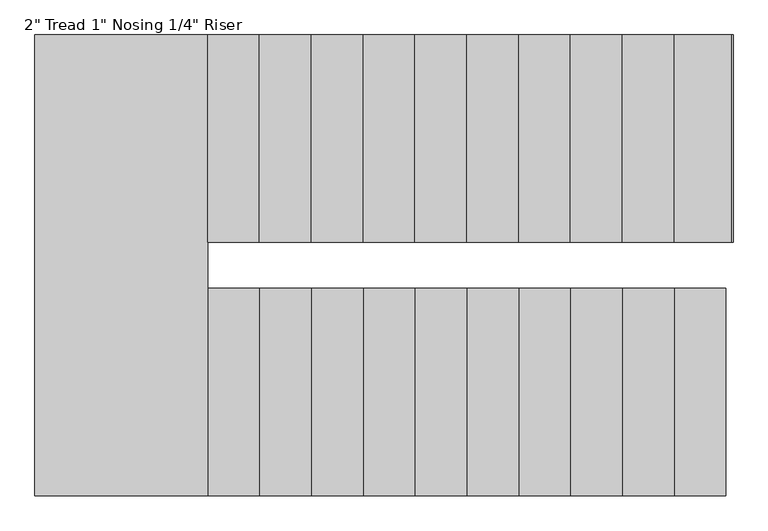
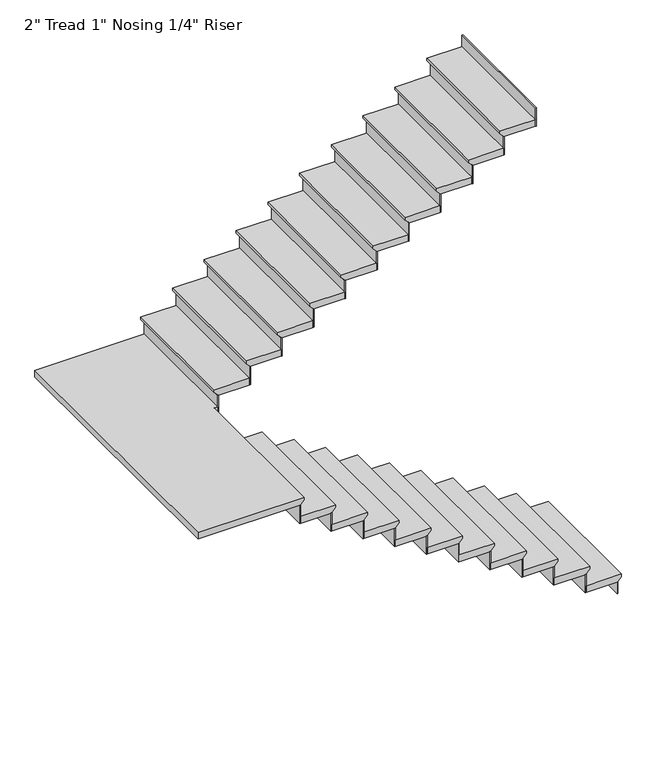
"""IFC4 building model written with IfcOpenShell, lengths in millimetres: stair flight geometry."""

from ifc_helpers import new_model, si_unit, origin, place, context, project, spatial, faceted_brep, source, transform, mapped, element, save


def stair_flight_418e8841(model_context):
    return source(origin(), model_context, "Body", "Brep", [
        faceted_brep([(-2080.8410855, 332.1803617, 12921.0954545), (-2080.8410855, 332.1803617, 12940.1454545), (-2080.8410855, -582.2196383, 12940.1454545), (-2080.8410855, -582.2196383, 12921.0954545), (-2106.2410855, 332.1803617, 12895.6954545), (-2106.2410855, -582.2196383, 12895.6954545), (-2334.8410855, 332.1803617, 12940.1454545), (-2334.8410855, -582.2196383, 12940.1454545), (-2106.2410855, -582.2196383, 12889.3454545), (-2334.8410855, -582.2196383, 12889.3454545), (-2334.8410855, 332.1803617, 12889.3454545), (-2106.2410855, 332.1803617, 12889.3454545)], [[[0, 1, 2, 3]], [[4, 0, 3, 5]], [[2, 1, 6, 7]], [[8, 9, 10, 11]], [[2, 7, 9, 8, 5, 3]], [[8, 11, 4, 5]], [[6, 1, 0, 4, 11, 10]], [[7, 6, 10, 9]]]),
        faceted_brep([(-2106.2410855, 332.1803617, 12889.3454545), (-2106.2410855, 332.1803617, 12801.6), (-2112.5910855, 332.1803617, 12801.6), (-2112.5910855, 332.1803617, 12889.3454545), (-2106.2410855, -582.2196383, 12889.3454545), (-2112.5910855, -582.2196383, 12889.3454545), (-2112.5910855, -582.2196383, 12801.6), (-2106.2410855, -582.2196383, 12801.6)], [[[0, 1, 2, 3]], [[4, 5, 6, 7]], [[1, 0, 4, 7]], [[2, 1, 7, 6]], [[3, 2, 6, 5]], [[0, 3, 5, 4]]]),
        faceted_brep([(-2334.8410855, 332.1803617, 13027.8909091), (-2334.8410855, 332.1803617, 12889.3454545), (-2341.1910855, 332.1803617, 12889.3454545), (-2341.1910855, 332.1803617, 13027.8909091), (-2334.8410855, -582.2196383, 13027.8909091), (-2341.1910855, -582.2196383, 13027.8909091), (-2341.1910855, -582.2196383, 12889.3454545), (-2334.8410855, -582.2196383, 12889.3454545)], [[[0, 1, 2, 3]], [[4, 5, 6, 7]], [[1, 0, 4, 7]], [[2, 1, 7, 6]], [[3, 2, 6, 5]], [[0, 3, 5, 4]]]),
        faceted_brep([(-2309.4410855, -582.2196383, 13078.6909091), (-2309.4410855, 332.1803617, 13078.6909091), (-2563.4410855, 332.1803617, 13078.6909091), (-2563.4410855, -582.2196383, 13078.6909091), (-2334.8410855, -582.2196383, 13027.8909091), (-2563.4410855, -582.2196383, 13027.8909091), (-2563.4410855, 332.1803617, 13027.8909091), (-2334.8410855, 332.1803617, 13027.8909091), (-2334.8410855, -582.2196383, 13034.2409091), (-2309.4410855, -582.2196383, 13059.6409091), (-2334.8410855, 332.1803617, 13034.2409091), (-2309.4410855, 332.1803617, 13059.6409091)], [[[0, 1, 2, 3]], [[4, 5, 6, 7]], [[0, 3, 5, 4, 8, 9]], [[4, 7, 10, 8]], [[2, 1, 11, 10, 7, 6]], [[3, 2, 6, 5]], [[11, 1, 0, 9]], [[10, 11, 9, 8]]]),
        faceted_brep([(-2563.4410855, 332.1803617, 13166.4363636), (-2563.4410855, 332.1803617, 13027.8909091), (-2569.7910855, 332.1803617, 13027.8909091), (-2569.7910855, 332.1803617, 13166.4363636), (-2563.4410855, -582.2196383, 13166.4363636), (-2569.7910855, -582.2196383, 13166.4363636), (-2569.7910855, -582.2196383, 13027.8909091), (-2563.4410855, -582.2196383, 13027.8909091)], [[[0, 1, 2, 3]], [[4, 5, 6, 7]], [[1, 0, 4, 7]], [[2, 1, 7, 6]], [[3, 2, 6, 5]], [[0, 3, 5, 4]]]),
        faceted_brep([(-2538.0410855, -582.2196383, 13217.2363636), (-2538.0410855, 332.1803617, 13217.2363636), (-2792.0410855, 332.1803617, 13217.2363636), (-2792.0410855, -582.2196383, 13217.2363636), (-2563.4410855, -582.2196383, 13166.4363636), (-2792.0410855, -582.2196383, 13166.4363636), (-2792.0410855, 332.1803617, 13166.4363636), (-2563.4410855, 332.1803617, 13166.4363636), (-2563.4410855, -582.2196383, 13172.7863636), (-2538.0410855, -582.2196383, 13198.1863636), (-2563.4410855, 332.1803617, 13172.7863636), (-2538.0410855, 332.1803617, 13198.1863636)], [[[0, 1, 2, 3]], [[4, 5, 6, 7]], [[0, 3, 5, 4, 8, 9]], [[4, 7, 10, 8]], [[2, 1, 11, 10, 7, 6]], [[3, 2, 6, 5]], [[11, 1, 0, 9]], [[10, 11, 9, 8]]]),
        faceted_brep([(-2792.0410855, 332.1803617, 13304.9818182), (-2792.0410855, 332.1803617, 13166.4363636), (-2798.3910855, 332.1803617, 13166.4363636), (-2798.3910855, 332.1803617, 13304.9818182), (-2792.0410855, -582.2196383, 13304.9818182), (-2798.3910855, -582.2196383, 13304.9818182), (-2798.3910855, -582.2196383, 13166.4363636), (-2792.0410855, -582.2196383, 13166.4363636)], [[[0, 1, 2, 3]], [[4, 5, 6, 7]], [[1, 0, 4, 7]], [[2, 1, 7, 6]], [[3, 2, 6, 5]], [[0, 3, 5, 4]]]),
        faceted_brep([(-2766.6410855, -582.2196383, 13355.7818182), (-2766.6410855, 332.1803617, 13355.7818182), (-3020.6410855, 332.1803617, 13355.7818182), (-3020.6410855, -582.2196383, 13355.7818182), (-2792.0410855, -582.2196383, 13304.9818182), (-3020.6410855, -582.2196383, 13304.9818182), (-3020.6410855, 332.1803617, 13304.9818182), (-2792.0410855, 332.1803617, 13304.9818182), (-2792.0410855, -582.2196383, 13311.3318182), (-2766.6410855, -582.2196383, 13336.7318182), (-2792.0410855, 332.1803617, 13311.3318182), (-2766.6410855, 332.1803617, 13336.7318182)], [[[0, 1, 2, 3]], [[4, 5, 6, 7]], [[0, 3, 5, 4, 8, 9]], [[4, 7, 10, 8]], [[2, 1, 11, 10, 7, 6]], [[3, 2, 6, 5]], [[11, 1, 0, 9]], [[10, 11, 9, 8]]]),
        faceted_brep([(-3020.6410855, 332.1803617, 13443.5272727), (-3020.6410855, 332.1803617, 13304.9818182), (-3026.9910855, 332.1803617, 13304.9818182), (-3026.9910855, 332.1803617, 13443.5272727), (-3020.6410855, -582.2196383, 13443.5272727), (-3026.9910855, -582.2196383, 13443.5272727), (-3026.9910855, -582.2196383, 13304.9818182), (-3020.6410855, -582.2196383, 13304.9818182)], [[[0, 1, 2, 3]], [[4, 5, 6, 7]], [[1, 0, 4, 7]], [[2, 1, 7, 6]], [[3, 2, 6, 5]], [[0, 3, 5, 4]]]),
        faceted_brep([(-2995.2410855, -582.2196383, 13494.3272727), (-2995.2410855, 332.1803617, 13494.3272727), (-3249.2410855, 332.1803617, 13494.3272727), (-3249.2410855, -582.2196383, 13494.3272727), (-3020.6410855, -582.2196383, 13443.5272727), (-3249.2410855, -582.2196383, 13443.5272727), (-3249.2410855, 332.1803617, 13443.5272727), (-3020.6410855, 332.1803617, 13443.5272727), (-3020.6410855, -582.2196383, 13449.8772727), (-2995.2410855, -582.2196383, 13475.2772727), (-3020.6410855, 332.1803617, 13449.8772727), (-2995.2410855, 332.1803617, 13475.2772727)], [[[0, 1, 2, 3]], [[4, 5, 6, 7]], [[0, 3, 5, 4, 8, 9]], [[4, 7, 10, 8]], [[2, 1, 11, 10, 7, 6]], [[3, 2, 6, 5]], [[11, 1, 0, 9]], [[10, 11, 9, 8]]]),
        faceted_brep([(-3249.2410855, 332.1803617, 13582.0727273), (-3249.2410855, 332.1803617, 13443.5272727), (-3255.5910855, 332.1803617, 13443.5272727), (-3255.5910855, 332.1803617, 13582.0727273), (-3249.2410855, -582.2196383, 13582.0727273), (-3255.5910855, -582.2196383, 13582.0727273), (-3255.5910855, -582.2196383, 13443.5272727), (-3249.2410855, -582.2196383, 13443.5272727)], [[[0, 1, 2, 3]], [[4, 5, 6, 7]], [[1, 0, 4, 7]], [[2, 1, 7, 6]], [[3, 2, 6, 5]], [[0, 3, 5, 4]]]),
        faceted_brep([(-3223.8410855, -582.2196383, 13632.8727273), (-3223.8410855, 332.1803617, 13632.8727273), (-3477.8410855, 332.1803617, 13632.8727273), (-3477.8410855, -582.2196383, 13632.8727273), (-3249.2410855, -582.2196383, 13582.0727273), (-3477.8410855, -582.2196383, 13582.0727273), (-3477.8410855, 332.1803617, 13582.0727273), (-3249.2410855, 332.1803617, 13582.0727273), (-3249.2410855, -582.2196383, 13588.4227273), (-3223.8410855, -582.2196383, 13613.8227273), (-3249.2410855, 332.1803617, 13588.4227273), (-3223.8410855, 332.1803617, 13613.8227273)], [[[0, 1, 2, 3]], [[4, 5, 6, 7]], [[0, 3, 5, 4, 8, 9]], [[4, 7, 10, 8]], [[2, 1, 11, 10, 7, 6]], [[3, 2, 6, 5]], [[11, 1, 0, 9]], [[10, 11, 9, 8]]]),
        faceted_brep([(-3477.8410855, 332.1803617, 13720.6181818), (-3477.8410855, 332.1803617, 13582.0727273), (-3484.1910855, 332.1803617, 13582.0727273), (-3484.1910855, 332.1803617, 13720.6181818), (-3477.8410855, -582.2196383, 13720.6181818), (-3484.1910855, -582.2196383, 13720.6181818), (-3484.1910855, -582.2196383, 13582.0727273), (-3477.8410855, -582.2196383, 13582.0727273)], [[[0, 1, 2, 3]], [[4, 5, 6, 7]], [[1, 0, 4, 7]], [[2, 1, 7, 6]], [[3, 2, 6, 5]], [[0, 3, 5, 4]]]),
        faceted_brep([(-3452.4410855, -582.2196383, 13771.4181818), (-3452.4410855, 332.1803617, 13771.4181818), (-3706.4410855, 332.1803617, 13771.4181818), (-3706.4410855, -582.2196383, 13771.4181818), (-3477.8410855, -582.2196383, 13720.6181818), (-3706.4410855, -582.2196383, 13720.6181818), (-3706.4410855, 332.1803617, 13720.6181818), (-3477.8410855, 332.1803617, 13720.6181818), (-3477.8410855, -582.2196383, 13726.9681818), (-3452.4410855, -582.2196383, 13752.3681818), (-3477.8410855, 332.1803617, 13726.9681818), (-3452.4410855, 332.1803617, 13752.3681818)], [[[0, 1, 2, 3]], [[4, 5, 6, 7]], [[0, 3, 5, 4, 8, 9]], [[4, 7, 10, 8]], [[2, 1, 11, 10, 7, 6]], [[3, 2, 6, 5]], [[11, 1, 0, 9]], [[10, 11, 9, 8]]]),
        faceted_brep([(-3706.4410855, 332.1803617, 13859.1636364), (-3706.4410855, 332.1803617, 13720.6181818), (-3712.7910855, 332.1803617, 13720.6181818), (-3712.7910855, 332.1803617, 13859.1636364), (-3706.4410855, -582.2196383, 13859.1636364), (-3712.7910855, -582.2196383, 13859.1636364), (-3712.7910855, -582.2196383, 13720.6181818), (-3706.4410855, -582.2196383, 13720.6181818)], [[[0, 1, 2, 3]], [[4, 5, 6, 7]], [[1, 0, 4, 7]], [[2, 1, 7, 6]], [[3, 2, 6, 5]], [[0, 3, 5, 4]]]),
        faceted_brep([(-3681.0410855, -582.2196383, 13909.9636364), (-3681.0410855, 332.1803617, 13909.9636364), (-3935.0410855, 332.1803617, 13909.9636364), (-3935.0410855, -582.2196383, 13909.9636364), (-3706.4410855, -582.2196383, 13859.1636364), (-3935.0410855, -582.2196383, 13859.1636364), (-3935.0410855, 332.1803617, 13859.1636364), (-3706.4410855, 332.1803617, 13859.1636364), (-3706.4410855, -582.2196383, 13865.5136364), (-3681.0410855, -582.2196383, 13890.9136364), (-3706.4410855, 332.1803617, 13865.5136364), (-3681.0410855, 332.1803617, 13890.9136364)], [[[0, 1, 2, 3]], [[4, 5, 6, 7]], [[0, 3, 5, 4, 8, 9]], [[4, 7, 10, 8]], [[2, 1, 11, 10, 7, 6]], [[3, 2, 6, 5]], [[11, 1, 0, 9]], [[10, 11, 9, 8]]]),
        faceted_brep([(-3935.0410855, 332.1803617, 13997.7090909), (-3935.0410855, 332.1803617, 13859.1636364), (-3941.3910855, 332.1803617, 13859.1636364), (-3941.3910855, 332.1803617, 13997.7090909), (-3935.0410855, -582.2196383, 13997.7090909), (-3941.3910855, -582.2196383, 13997.7090909), (-3941.3910855, -582.2196383, 13859.1636364), (-3935.0410855, -582.2196383, 13859.1636364)], [[[0, 1, 2, 3]], [[4, 5, 6, 7]], [[1, 0, 4, 7]], [[2, 1, 7, 6]], [[3, 2, 6, 5]], [[0, 3, 5, 4]]]),
        faceted_brep([(-3909.6410855, -582.2196383, 14048.5090909), (-3909.6410855, 332.1803617, 14048.5090909), (-4163.6410855, 332.1803617, 14048.5090909), (-4163.6410855, -582.2196383, 14048.5090909), (-3935.0410855, -582.2196383, 13997.7090909), (-4163.6410855, -582.2196383, 13997.7090909), (-4163.6410855, 332.1803617, 13997.7090909), (-3935.0410855, 332.1803617, 13997.7090909), (-3935.0410855, -582.2196383, 14004.0590909), (-3909.6410855, -582.2196383, 14029.4590909), (-3935.0410855, 332.1803617, 14004.0590909), (-3909.6410855, 332.1803617, 14029.4590909)], [[[0, 1, 2, 3]], [[4, 5, 6, 7]], [[0, 3, 5, 4, 8, 9]], [[4, 7, 10, 8]], [[2, 1, 11, 10, 7, 6]], [[3, 2, 6, 5]], [[11, 1, 0, 9]], [[10, 11, 9, 8]]]),
        faceted_brep([(-4163.6410855, 332.1803617, 14136.2545455), (-4163.6410855, 332.1803617, 13997.7090909), (-4169.9910855, 332.1803617, 13997.7090909), (-4169.9910855, 332.1803617, 14136.2545455), (-4163.6410855, -582.2196383, 14136.2545455), (-4169.9910855, -582.2196383, 14136.2545455), (-4169.9910855, -582.2196383, 13997.7090909), (-4163.6410855, -582.2196383, 13997.7090909)], [[[0, 1, 2, 3]], [[4, 5, 6, 7]], [[1, 0, 4, 7]], [[2, 1, 7, 6]], [[3, 2, 6, 5]], [[0, 3, 5, 4]]]),
        faceted_brep([(-4138.2410855, -582.2196383, 14187.0545455), (-4138.2410855, 332.1803617, 14187.0545455), (-4392.2410855, 332.1803617, 14187.0545455), (-4392.2410855, -582.2196383, 14187.0545455), (-4163.6410855, -582.2196383, 14136.2545455), (-4392.2410855, -582.2196383, 14136.2545455), (-4392.2410855, 332.1803617, 14136.2545455), (-4163.6410855, 332.1803617, 14136.2545455), (-4163.6410855, -582.2196383, 14142.6045455), (-4138.2410855, -582.2196383, 14168.0045455), (-4163.6410855, 332.1803617, 14142.6045455), (-4138.2410855, 332.1803617, 14168.0045455)], [[[0, 1, 2, 3]], [[4, 5, 6, 7]], [[0, 3, 5, 4, 8, 9]], [[4, 7, 10, 8]], [[2, 1, 11, 10, 7, 6]], [[3, 2, 6, 5]], [[11, 1, 0, 9]], [[10, 11, 9, 8]]]),
        faceted_brep([(-4392.2410855, 332.1803617, 14274.8), (-4392.2410855, 332.1803617, 14136.2545455), (-4398.5910855, 332.1803617, 14136.2545455), (-4398.5910855, 332.1803617, 14274.8), (-4392.2410855, -582.2196383, 14274.8), (-4398.5910855, -582.2196383, 14274.8), (-4398.5910855, -582.2196383, 14136.2545455), (-4392.2410855, -582.2196383, 14136.2545455)], [[[0, 1, 2, 3]], [[4, 5, 6, 7]], [[1, 0, 4, 7]], [[2, 1, 7, 6]], [[3, 2, 6, 5]], [[0, 3, 5, 4]]]),
        faceted_brep([(-4341.4410855, 1449.7803617, 14325.6), (-5128.8410855, 1449.7803617, 14325.6), (-5128.8410855, -582.2196383, 14325.6), (-4366.8410855, -582.2196383, 14325.6), (-4366.8410855, 535.3803617, 14325.6), (-4341.4410855, 535.3803617, 14325.6), (-5128.8410855, 1449.7803617, 14274.8), (-4341.4410855, 1449.7803617, 14274.8), (-4341.4410855, 535.3803617, 14274.8), (-4366.8410855, 535.3803617, 14274.8), (-4366.8410855, 332.1803617, 14274.8), (-4392.2410855, 332.1803617, 14274.8), (-4392.2410855, -582.2196383, 14274.8), (-5128.8410855, -582.2196383, 14274.8), (-4392.2410855, -582.2196383, 14281.15), (-4366.8410855, -582.2196383, 14306.55), (-4392.2410855, 332.1803617, 14281.15), (-4366.8410855, 332.1803617, 14306.55)], [[[0, 1, 2, 3, 4, 5]], [[6, 7, 8, 9, 10, 11, 12, 13]], [[1, 0, 7, 6]], [[2, 1, 6, 13]], [[3, 2, 13, 12, 14, 15]], [[12, 11, 16, 14]], [[11, 10, 17, 16]], [[4, 3, 15, 17, 10, 9]], [[5, 4, 9, 8]], [[0, 5, 8, 7]], [[15, 14, 16, 17]]]),
        faceted_brep([(-4341.4410855, 535.3803617, 14413.3454545), (-4341.4410855, 535.3803617, 14274.8), (-4335.0910855, 535.3803617, 14274.8), (-4335.0910855, 535.3803617, 14413.3454545), (-4341.4410855, 1449.7803617, 14413.3454545), (-4335.0910855, 1449.7803617, 14413.3454545), (-4335.0910855, 1449.7803617, 14274.8), (-4341.4410855, 1449.7803617, 14274.8)], [[[0, 1, 2, 3]], [[4, 5, 6, 7]], [[1, 0, 4, 7]], [[2, 1, 7, 6]], [[3, 2, 6, 5]], [[0, 3, 5, 4]]]),
        faceted_brep([(-4366.8410855, 1449.7803617, 14464.1454545), (-4366.8410855, 535.3803617, 14464.1454545), (-4112.8410855, 535.3803617, 14464.1454545), (-4112.8410855, 1449.7803617, 14464.1454545), (-4341.4410855, 1449.7803617, 14413.3454545), (-4112.8410855, 1449.7803617, 14413.3454545), (-4112.8410855, 535.3803617, 14413.3454545), (-4341.4410855, 535.3803617, 14413.3454545), (-4341.4410855, 1449.7803617, 14419.6954545), (-4366.8410855, 1449.7803617, 14445.0954545), (-4341.4410855, 535.3803617, 14419.6954545), (-4366.8410855, 535.3803617, 14445.0954545)], [[[0, 1, 2, 3]], [[4, 5, 6, 7]], [[0, 3, 5, 4, 8, 9]], [[4, 7, 10, 8]], [[2, 1, 11, 10, 7, 6]], [[3, 2, 6, 5]], [[11, 1, 0, 9]], [[10, 11, 9, 8]]]),
        faceted_brep([(-4112.8410855, 535.3803617, 14551.8909091), (-4112.8410855, 535.3803617, 14413.3454545), (-4106.4910855, 535.3803617, 14413.3454545), (-4106.4910855, 535.3803617, 14551.8909091), (-4112.8410855, 1449.7803617, 14551.8909091), (-4106.4910855, 1449.7803617, 14551.8909091), (-4106.4910855, 1449.7803617, 14413.3454545), (-4112.8410855, 1449.7803617, 14413.3454545)], [[[0, 1, 2, 3]], [[4, 5, 6, 7]], [[1, 0, 4, 7]], [[2, 1, 7, 6]], [[3, 2, 6, 5]], [[0, 3, 5, 4]]]),
        faceted_brep([(-4138.2410855, 1449.7803617, 14602.6909091), (-4138.2410855, 535.3803617, 14602.6909091), (-3884.2410855, 535.3803617, 14602.6909091), (-3884.2410855, 1449.7803617, 14602.6909091), (-4112.8410855, 1449.7803617, 14551.8909091), (-3884.2410855, 1449.7803617, 14551.8909091), (-3884.2410855, 535.3803617, 14551.8909091), (-4112.8410855, 535.3803617, 14551.8909091), (-4112.8410855, 1449.7803617, 14558.2409091), (-4138.2410855, 1449.7803617, 14583.6409091), (-4112.8410855, 535.3803617, 14558.2409091), (-4138.2410855, 535.3803617, 14583.6409091)], [[[0, 1, 2, 3]], [[4, 5, 6, 7]], [[0, 3, 5, 4, 8, 9]], [[4, 7, 10, 8]], [[2, 1, 11, 10, 7, 6]], [[3, 2, 6, 5]], [[11, 1, 0, 9]], [[10, 11, 9, 8]]]),
        faceted_brep([(-3884.2410855, 535.3803617, 14690.4363636), (-3884.2410855, 535.3803617, 14551.8909091), (-3877.8910855, 535.3803617, 14551.8909091), (-3877.8910855, 535.3803617, 14690.4363636), (-3884.2410855, 1449.7803617, 14690.4363636), (-3877.8910855, 1449.7803617, 14690.4363636), (-3877.8910855, 1449.7803617, 14551.8909091), (-3884.2410855, 1449.7803617, 14551.8909091)], [[[0, 1, 2, 3]], [[4, 5, 6, 7]], [[1, 0, 4, 7]], [[2, 1, 7, 6]], [[3, 2, 6, 5]], [[0, 3, 5, 4]]]),
        faceted_brep([(-3909.6410855, 1449.7803617, 14741.2363636), (-3909.6410855, 535.3803617, 14741.2363636), (-3655.6410855, 535.3803617, 14741.2363636), (-3655.6410855, 1449.7803617, 14741.2363636), (-3884.2410855, 1449.7803617, 14690.4363636), (-3655.6410855, 1449.7803617, 14690.4363636), (-3655.6410855, 535.3803617, 14690.4363636), (-3884.2410855, 535.3803617, 14690.4363636), (-3884.2410855, 1449.7803617, 14696.7863636), (-3909.6410855, 1449.7803617, 14722.1863636), (-3884.2410855, 535.3803617, 14696.7863636), (-3909.6410855, 535.3803617, 14722.1863636)], [[[0, 1, 2, 3]], [[4, 5, 6, 7]], [[0, 3, 5, 4, 8, 9]], [[4, 7, 10, 8]], [[2, 1, 11, 10, 7, 6]], [[3, 2, 6, 5]], [[11, 1, 0, 9]], [[10, 11, 9, 8]]]),
        faceted_brep([(-3655.6410855, 535.3803617, 14828.9818182), (-3655.6410855, 535.3803617, 14690.4363636), (-3649.2910855, 535.3803617, 14690.4363636), (-3649.2910855, 535.3803617, 14828.9818182), (-3655.6410855, 1449.7803617, 14828.9818182), (-3649.2910855, 1449.7803617, 14828.9818182), (-3649.2910855, 1449.7803617, 14690.4363636), (-3655.6410855, 1449.7803617, 14690.4363636)], [[[0, 1, 2, 3]], [[4, 5, 6, 7]], [[1, 0, 4, 7]], [[2, 1, 7, 6]], [[3, 2, 6, 5]], [[0, 3, 5, 4]]]),
        faceted_brep([(-3681.0410855, 1449.7803617, 14879.7818182), (-3681.0410855, 535.3803617, 14879.7818182), (-3427.0410855, 535.3803617, 14879.7818182), (-3427.0410855, 1449.7803617, 14879.7818182), (-3655.6410855, 1449.7803617, 14828.9818182), (-3427.0410855, 1449.7803617, 14828.9818182), (-3427.0410855, 535.3803617, 14828.9818182), (-3655.6410855, 535.3803617, 14828.9818182), (-3655.6410855, 1449.7803617, 14835.3318182), (-3681.0410855, 1449.7803617, 14860.7318182), (-3655.6410855, 535.3803617, 14835.3318182), (-3681.0410855, 535.3803617, 14860.7318182)], [[[0, 1, 2, 3]], [[4, 5, 6, 7]], [[0, 3, 5, 4, 8, 9]], [[4, 7, 10, 8]], [[2, 1, 11, 10, 7, 6]], [[3, 2, 6, 5]], [[11, 1, 0, 9]], [[10, 11, 9, 8]]]),
        faceted_brep([(-3427.0410855, 535.3803617, 14967.5272727), (-3427.0410855, 535.3803617, 14828.9818182), (-3420.6910855, 535.3803617, 14828.9818182), (-3420.6910855, 535.3803617, 14967.5272727), (-3427.0410855, 1449.7803617, 14967.5272727), (-3420.6910855, 1449.7803617, 14967.5272727), (-3420.6910855, 1449.7803617, 14828.9818182), (-3427.0410855, 1449.7803617, 14828.9818182)], [[[0, 1, 2, 3]], [[4, 5, 6, 7]], [[1, 0, 4, 7]], [[2, 1, 7, 6]], [[3, 2, 6, 5]], [[0, 3, 5, 4]]]),
        faceted_brep([(-3452.4410855, 1449.7803617, 15018.3272727), (-3452.4410855, 535.3803617, 15018.3272727), (-3198.4410855, 535.3803617, 15018.3272727), (-3198.4410855, 1449.7803617, 15018.3272727), (-3427.0410855, 1449.7803617, 14967.5272727), (-3198.4410855, 1449.7803617, 14967.5272727), (-3198.4410855, 535.3803617, 14967.5272727), (-3427.0410855, 535.3803617, 14967.5272727), (-3427.0410855, 1449.7803617, 14973.8772727), (-3452.4410855, 1449.7803617, 14999.2772727), (-3427.0410855, 535.3803617, 14973.8772727), (-3452.4410855, 535.3803617, 14999.2772727)], [[[0, 1, 2, 3]], [[4, 5, 6, 7]], [[0, 3, 5, 4, 8, 9]], [[4, 7, 10, 8]], [[2, 1, 11, 10, 7, 6]], [[3, 2, 6, 5]], [[11, 1, 0, 9]], [[10, 11, 9, 8]]]),
        faceted_brep([(-3198.4410855, 535.3803617, 15106.0727273), (-3198.4410855, 535.3803617, 14967.5272727), (-3192.0910855, 535.3803617, 14967.5272727), (-3192.0910855, 535.3803617, 15106.0727273), (-3198.4410855, 1449.7803617, 15106.0727273), (-3192.0910855, 1449.7803617, 15106.0727273), (-3192.0910855, 1449.7803617, 14967.5272727), (-3198.4410855, 1449.7803617, 14967.5272727)], [[[0, 1, 2, 3]], [[4, 5, 6, 7]], [[1, 0, 4, 7]], [[2, 1, 7, 6]], [[3, 2, 6, 5]], [[0, 3, 5, 4]]]),
        faceted_brep([(-3223.8410855, 1449.7803617, 15156.8727273), (-3223.8410855, 535.3803617, 15156.8727273), (-2969.8410855, 535.3803617, 15156.8727273), (-2969.8410855, 1449.7803617, 15156.8727273), (-3198.4410855, 1449.7803617, 15106.0727273), (-2969.8410855, 1449.7803617, 15106.0727273), (-2969.8410855, 535.3803617, 15106.0727273), (-3198.4410855, 535.3803617, 15106.0727273), (-3198.4410855, 1449.7803617, 15112.4227273), (-3223.8410855, 1449.7803617, 15137.8227273), (-3198.4410855, 535.3803617, 15112.4227273), (-3223.8410855, 535.3803617, 15137.8227273)], [[[0, 1, 2, 3]], [[4, 5, 6, 7]], [[0, 3, 5, 4, 8, 9]], [[4, 7, 10, 8]], [[2, 1, 11, 10, 7, 6]], [[3, 2, 6, 5]], [[11, 1, 0, 9]], [[10, 11, 9, 8]]]),
        faceted_brep([(-2969.8410855, 535.3803617, 15244.6181818), (-2969.8410855, 535.3803617, 15106.0727273), (-2963.4910855, 535.3803617, 15106.0727273), (-2963.4910855, 535.3803617, 15244.6181818), (-2969.8410855, 1449.7803617, 15244.6181818), (-2963.4910855, 1449.7803617, 15244.6181818), (-2963.4910855, 1449.7803617, 15106.0727273), (-2969.8410855, 1449.7803617, 15106.0727273)], [[[0, 1, 2, 3]], [[4, 5, 6, 7]], [[1, 0, 4, 7]], [[2, 1, 7, 6]], [[3, 2, 6, 5]], [[0, 3, 5, 4]]]),
        faceted_brep([(-2995.2410855, 1449.7803617, 15295.4181818), (-2995.2410855, 535.3803617, 15295.4181818), (-2741.2410855, 535.3803617, 15295.4181818), (-2741.2410855, 1449.7803617, 15295.4181818), (-2969.8410855, 1449.7803617, 15244.6181818), (-2741.2410855, 1449.7803617, 15244.6181818), (-2741.2410855, 535.3803617, 15244.6181818), (-2969.8410855, 535.3803617, 15244.6181818), (-2969.8410855, 1449.7803617, 15250.9681818), (-2995.2410855, 1449.7803617, 15276.3681818), (-2969.8410855, 535.3803617, 15250.9681818), (-2995.2410855, 535.3803617, 15276.3681818)], [[[0, 1, 2, 3]], [[4, 5, 6, 7]], [[0, 3, 5, 4, 8, 9]], [[4, 7, 10, 8]], [[2, 1, 11, 10, 7, 6]], [[3, 2, 6, 5]], [[11, 1, 0, 9]], [[10, 11, 9, 8]]]),
        faceted_brep([(-2741.2410855, 535.3803617, 15383.1636364), (-2741.2410855, 535.3803617, 15244.6181818), (-2734.8910855, 535.3803617, 15244.6181818), (-2734.8910855, 535.3803617, 15383.1636364), (-2741.2410855, 1449.7803617, 15383.1636364), (-2734.8910855, 1449.7803617, 15383.1636364), (-2734.8910855, 1449.7803617, 15244.6181818), (-2741.2410855, 1449.7803617, 15244.6181818)], [[[0, 1, 2, 3]], [[4, 5, 6, 7]], [[1, 0, 4, 7]], [[2, 1, 7, 6]], [[3, 2, 6, 5]], [[0, 3, 5, 4]]]),
        faceted_brep([(-2766.6410855, 1449.7803617, 15433.9636364), (-2766.6410855, 535.3803617, 15433.9636364), (-2512.6410855, 535.3803617, 15433.9636364), (-2512.6410855, 1449.7803617, 15433.9636364), (-2741.2410855, 1449.7803617, 15383.1636364), (-2512.6410855, 1449.7803617, 15383.1636364), (-2512.6410855, 535.3803617, 15383.1636364), (-2741.2410855, 535.3803617, 15383.1636364), (-2741.2410855, 1449.7803617, 15389.5136364), (-2766.6410855, 1449.7803617, 15414.9136364), (-2741.2410855, 535.3803617, 15389.5136364), (-2766.6410855, 535.3803617, 15414.9136364)], [[[0, 1, 2, 3]], [[4, 5, 6, 7]], [[0, 3, 5, 4, 8, 9]], [[4, 7, 10, 8]], [[2, 1, 11, 10, 7, 6]], [[3, 2, 6, 5]], [[11, 1, 0, 9]], [[10, 11, 9, 8]]]),
        faceted_brep([(-2512.6410855, 535.3803617, 15521.7090909), (-2512.6410855, 535.3803617, 15383.1636364), (-2506.2910855, 535.3803617, 15383.1636364), (-2506.2910855, 535.3803617, 15521.7090909), (-2512.6410855, 1449.7803617, 15521.7090909), (-2506.2910855, 1449.7803617, 15521.7090909), (-2506.2910855, 1449.7803617, 15383.1636364), (-2512.6410855, 1449.7803617, 15383.1636364)], [[[0, 1, 2, 3]], [[4, 5, 6, 7]], [[1, 0, 4, 7]], [[2, 1, 7, 6]], [[3, 2, 6, 5]], [[0, 3, 5, 4]]]),
        faceted_brep([(-2538.0410855, 1449.7803617, 15572.5090909), (-2538.0410855, 535.3803617, 15572.5090909), (-2284.0410855, 535.3803617, 15572.5090909), (-2284.0410855, 1449.7803617, 15572.5090909), (-2512.6410855, 1449.7803617, 15521.7090909), (-2284.0410855, 1449.7803617, 15521.7090909), (-2284.0410855, 535.3803617, 15521.7090909), (-2512.6410855, 535.3803617, 15521.7090909), (-2512.6410855, 1449.7803617, 15528.0590909), (-2538.0410855, 1449.7803617, 15553.4590909), (-2512.6410855, 535.3803617, 15528.0590909), (-2538.0410855, 535.3803617, 15553.4590909)], [[[0, 1, 2, 3]], [[4, 5, 6, 7]], [[0, 3, 5, 4, 8, 9]], [[4, 7, 10, 8]], [[2, 1, 11, 10, 7, 6]], [[3, 2, 6, 5]], [[11, 1, 0, 9]], [[10, 11, 9, 8]]]),
        faceted_brep([(-2284.0410855, 535.3803617, 15660.2545455), (-2284.0410855, 535.3803617, 15521.7090909), (-2277.6910855, 535.3803617, 15521.7090909), (-2277.6910855, 535.3803617, 15660.2545455), (-2284.0410855, 1449.7803617, 15660.2545455), (-2277.6910855, 1449.7803617, 15660.2545455), (-2277.6910855, 1449.7803617, 15521.7090909), (-2284.0410855, 1449.7803617, 15521.7090909)], [[[0, 1, 2, 3]], [[4, 5, 6, 7]], [[1, 0, 4, 7]], [[2, 1, 7, 6]], [[3, 2, 6, 5]], [[0, 3, 5, 4]]]),
        faceted_brep([(-2055.4410855, 535.3803617, 15798.8), (-2055.4410855, 535.3803617, 15660.2545455), (-2049.0910855, 535.3803617, 15660.2545455), (-2049.0910855, 535.3803617, 15798.8), (-2055.4410855, 1449.7803617, 15798.8), (-2049.0910855, 1449.7803617, 15798.8), (-2049.0910855, 1449.7803617, 15660.2545455), (-2055.4410855, 1449.7803617, 15660.2545455)], [[[0, 1, 2, 3]], [[4, 5, 6, 7]], [[1, 0, 4, 7]], [[2, 1, 7, 6]], [[3, 2, 6, 5]], [[0, 3, 5, 4]]]),
        faceted_brep([(-2309.4410855, 1449.7803617, 15711.0545455), (-2309.4410855, 535.3803617, 15711.0545455), (-2055.4410855, 535.3803617, 15711.0545455), (-2055.4410855, 1449.7803617, 15711.0545455), (-2284.0410855, 1449.7803617, 15660.2545455), (-2055.4410855, 1449.7803617, 15660.2545455), (-2055.4410855, 535.3803617, 15660.2545455), (-2284.0410855, 535.3803617, 15660.2545455), (-2284.0410855, 1449.7803617, 15666.6045455), (-2309.4410855, 1449.7803617, 15692.0045455), (-2284.0410855, 535.3803617, 15666.6045455), (-2309.4410855, 535.3803617, 15692.0045455)], [[[0, 1, 2, 3]], [[4, 5, 6, 7]], [[0, 3, 5, 4, 8, 9]], [[4, 7, 10, 8]], [[2, 1, 11, 10, 7, 6]], [[3, 2, 6, 5]], [[11, 1, 0, 9]], [[10, 11, 9, 8]]]),
    ])


if __name__ == "__main__":
    model = new_model("IFC4")
    model_context = context("Model", 3, world=origin())
    ifc_project = project(units=[si_unit("LENGTHUNIT", "METRE", prefix="MILLI")], contexts=[model_context])
    site = spatial("IfcSite", under=ifc_project)
    building = spatial("IfcBuilding", under=site)
    placement = place(None, origin())
    stair_flight_shape = stair_flight_418e8841(model_context)
    element("IfcStairFlight", 1, ObjectType="2\" Tread 1\" Nosing 1/4\" Riser", at=placement, inside=building, context=model_context, shape_type="MappedRepresentation", body=[
        mapped(stair_flight_shape, transform((0.0, 0.0, 0.0), x_axis=(1.0, 0.0, 0.0), y_axis=(0.0, 1.0, 0.0), z_axis=(0.0, 0.0, 1.0))),
    ])
    save(model, "model.ifc")
